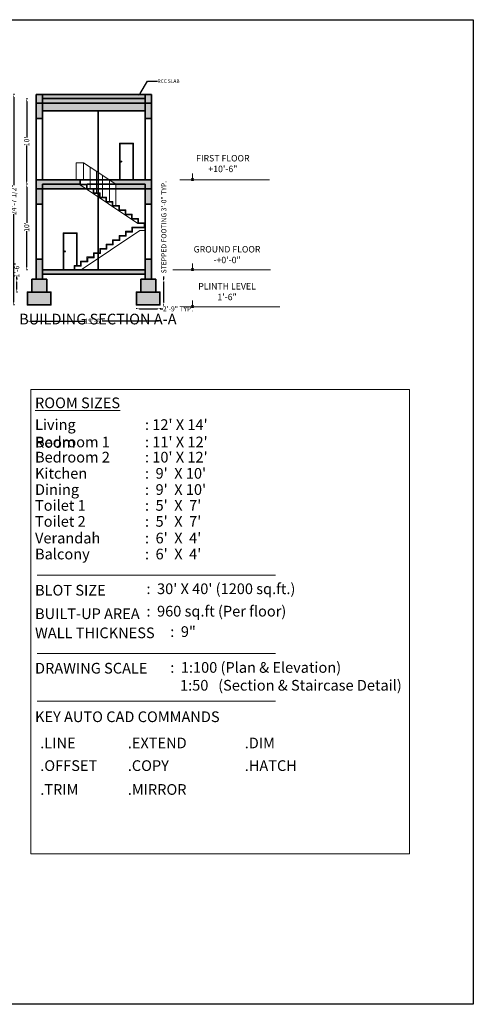
# Model space of a CAD drawing. Units: inches. Extents: x -80 to 1461, y -1239 to 153.
# Tile 6 of 6: x 824 to 1461, y -1239 to 141. Entities that reach past the tile are written whole.
import ezdxf
from ezdxf import colors
from ezdxf.entities.mleader import LeaderData, LeaderLine
from ezdxf.math import Vec2, Vec3

# ---------------------------------------------------------------- set-up
doc = ezdxf.new("R2010")
doc.units = ezdxf.units.IN
doc.header["$MEASUREMENT"] = 0
for name, color, linetype, lineweight in [('A-ANNO-DIMS', 2, 'Continuous', 18), ('A-ANNO-SYMB', 3, 'Continuous', 18), ('A-ANNO-TEXT', 7, 'Continuous', 18), ('A-ANNO-TTLB', 7, 'Continuous', 25), ('A-SECT', 7, 'Continuous', 35), ('A-SECT-PATT', 8, 'Continuous', 13), ('A-SECT-STRS', 7, 'Continuous', 20), ('DOOR', 32, 'Continuous', 18), ('S-FNDN', 7, 'Continuous', 35)]:
    doc.layers.add(name, color=color, linetype=linetype, lineweight=lineweight)
doc.styles.get("Standard").update_dxf_attribs({"font": 'arial.ttf'})
doc.dimstyles.get("Standard").update_dxf_attribs({"dimtxt": 7, "dimasz": 4, "dimexe": 0.18, "dimexo": 0.0625, "dimgap": 0.09, "dimtad": 0, "dimdec": 0, "dimzin": 0, "dimdsep": 46, "dimlunit": 3, "dimtxsty": 'Standard', "dimcen": 0.09, "dimadec": 0, "dimazin": 0, "dimtfac": 1, "dimtdec": 0, "dimtofl": 0, "dimtmove": 0, "dimatfit": 3, "dimfxl": 1, "dimfxlon": 1, "dimtolj": 1, "dimtzin": 0, "dimarcsym": 0})
pattern_1 = [(50, (-94.887, 315.974), (7.172602, -0.62752), [0.75, -8.25]), (355, (-94.887, 315.974), (-1.387513, 7.52192), [0.6, -6.6]), (100.45144, (-94.289, 315.9216), (5.78509, 6.8944), [0.6374, -7.01142]), (46.1842, (-94.887, 317.974), (10.672413, -1.65519), [1.125, -12.375]), (96.6356, (-93.998, 317.836), (9.34662, 9.74119), [0.9561, -10.51714]), (351.1842, (-94.887, 317.974), (9.34662, 9.74119), [0.9, -9.9]), (21, (-93.887, 317.474), (5.96907, -4.02619), [0.75, -8.25]), (326, (-93.887, 317.474), (2.433153, 7.2515), [0.6, -6.6]), (71.45144, (-93.3895, 317.1384), (8.402224, 3.22531), [0.6374, -7.01142]), (37.5, (-94.887, 315.974), (0.1215986, 3.3289385), [0, -6.52, 0, -6.7, 0, -6.625]), (7.5, (-94.887, 315.974), (2.630695, 3.944117), [0, -3.82, 0, -6.37, 0, -2.525]), (327.5, (-97.117, 315.974), (5.3382244, -0.225549), [0, -2.5, 0, -7.8, 0, -10.35]), (317.5, (-98.117, 315.974), (5.831862, 1.00105), [0, -3.25, 0, -5.18, 0, -7.35])]

# ---------------------------------------------------------------- blocks, each defined once
blk = doc.blocks.new('*D21')
at = {"layer": 'A-ANNO-DIMS', "color": 0, "lineweight": -2, "transparency": 16777216}
for p, q in [((820.2, -222.7), (820.2, -218.7)), ((821.2, -222.7), (820, -222.7)), ((820.2, -236.7), (820.2, -226.7)), ((821.2, -240.7), (820, -240.7))]:
    blk.add_line(p, q, dxfattribs=at)
at = {"layer": 'A-ANNO-DIMS', "color": 0, "transparency": 16777216}
for points in [[(819.5, -226.7), (820.9, -226.7), (820.2, -222.7)], [(819.5, -236.7), (820.9, -236.7), (820.2, -240.7)]]:
    blk.add_solid(points, dxfattribs=at)
at = {"layer": 'Defpoints', "color": 0, "transparency": 16777216}
for p in [(820.2, -222.7), (841.3, -222.7), (838.3, -240.7)]:
    blk.add_point(p, dxfattribs=at)
at = {"layer": 'A-ANNO-DIMS', "color": 0, "transparency": 16777216, "insert": (820.2, -209.6), "char_height": 7, "attachment_point": 5, "rotation": 90}
blk.add_mtext('\\A1;1\'-6"', dxfattribs=at)
blk = doc.blocks.new('*D22')
at = {"layer": 'A-ANNO-DIMS', "color": 0, "lineweight": -2, "transparency": 16777216}
for p, q in [((835.2, -89.4), (834, -89.4)), ((834.2, -93.4), (834.2, -143.7)), ((834.2, -205.4), (834.2, -155.1)), ((835.2, -209.4), (834, -209.4))]:
    blk.add_line(p, q, dxfattribs=at)
at = {"layer": 'A-ANNO-DIMS', "color": 0, "transparency": 16777216}
for points in [[(833.5, -93.4), (834.9, -93.4), (834.2, -89.4)], [(833.5, -205.4), (834.9, -205.4), (834.2, -209.4)]]:
    blk.add_solid(points, dxfattribs=at)
at = {"layer": 'Defpoints', "color": 0, "transparency": 16777216}
for p in [(834.2, -89.4), (856.3, -89.4), (856.3, -209.4)]:
    blk.add_point(p, dxfattribs=at)
at = {"layer": 'A-ANNO-DIMS', "color": 0, "transparency": 16777216, "insert": (834.2, -149.4), "char_height": 7, "attachment_point": 5, "rotation": 90}
blk.add_mtext("\\A1;10'", dxfattribs=at)
blk = doc.blocks.new('*D23')
at = {"layer": 'A-ANNO-DIMS', "color": 0, "lineweight": -2, "transparency": 16777216}
for p, q in [((835.2, 30.6), (834, 30.6)), ((834.2, 26.6), (834.2, -23.7)), ((834.2, -85.4), (834.2, -35.1)), ((835.2, -89.4), (834, -89.4))]:
    blk.add_line(p, q, dxfattribs=at)
at = {"layer": 'A-ANNO-DIMS', "color": 0, "transparency": 16777216}
for points in [[(833.5, 26.6), (834.9, 26.6), (834.2, 30.6)], [(833.5, -85.4), (834.9, -85.4), (834.2, -89.4)]]:
    blk.add_solid(points, dxfattribs=at)
at = {"layer": 'Defpoints', "color": 0, "transparency": 16777216}
for p in [(834.2, 30.6), (856.3, 30.6), (856.3, -89.4)]:
    blk.add_point(p, dxfattribs=at)
at = {"layer": 'A-ANNO-DIMS', "color": 0, "transparency": 16777216, "insert": (834.2, -29.4), "char_height": 7, "attachment_point": 5, "rotation": 90}
blk.add_mtext("\\A1;10'", dxfattribs=at)
blk = doc.blocks.new('FOOTING-STEPPED-SECTION')
blk.add_line((27, 36), (6, 36))
for points in [[(6, 36), (6, 18), (0, 18), (0, 0), (27, 0), (33, 0), (33, 18), (27, 18), (27, 36)], [(6, 18), (21, 18), (27, 18)]]:
    blk.add_lwpolyline(points)
blk = doc.blocks.new('LEVEL-DATUM')
h = blk.add_hatch(color=256)
h.dxf.hatch_style = 1
h.paths.add_polyline_path([(1.4, 2.8), (0, 2.8), (1.4, 1)])
h.paths.add_polyline_path([(2.8, 2.8), (1.4, 2.8), (1.4, 1)])
h = blk.add_hatch(color=256)
h.dxf.hatch_style = 1
h.paths.add_polyline_path([(2.8, 0), (2.8, 1), (0, 1), (0, 0)])
for p, q in [((1.4, 1), (0, 2.8)), ((0, 2.8), (1.4, 2.8)), ((0, 1), (2.8, 1)), ((0, 0), (0, 1)), ((2.8, 0), (0, 0)), ((1.4, 1), (1.4, 9.9)), ((1.4, 1), (2.8, 2.8)), ((2.8, 2.8), (1.4, 2.8)), ((2.8, 1), (2.8, 0))]:
    blk.add_line(p, q)
blk = doc.blocks.new('*D58')
at = {"layer": 'A-ANNO-DIMS', "color": 0, "lineweight": -2, "transparency": 16777216}
for p, q in [((1026.7, -222.7), (1026.7, -218.7)), ((1025.7, -222.7), (1026.8, -222.7)), ((1026.7, -254.7), (1026.7, -226.7)), ((1025.7, -258.7), (1026.8, -258.7))]:
    blk.add_line(p, q, dxfattribs=at)
at = {"layer": 'A-ANNO-DIMS', "color": 0, "transparency": 16777216}
for points in [[(1026, -226.7), (1027.3, -226.7), (1026.7, -222.7)], [(1026, -254.7), (1027.3, -254.7), (1026.7, -258.7)]]:
    blk.add_solid(points, dxfattribs=at)
at = {"layer": 'Defpoints', "color": 0, "transparency": 16777216}
for p in [(1021.3, -222.7), (1026.7, -222.7), (1021.3, -258.7)]:
    blk.add_point(p, dxfattribs=at)
at = {"layer": 'A-ANNO-DIMS', "color": 0, "transparency": 16777216, "insert": (1026.7, -149.5), "char_height": 7, "attachment_point": 5, "rotation": 90}
blk.add_mtext('\\A1;STEPPED FOOTING 3\'-0" TYP.', dxfattribs=at)
blk = doc.blocks.new('*D59')
at = {"layer": 'A-ANNO-DIMS', "color": 0, "lineweight": -2, "transparency": 16777216}
for p, q in [((988.3, -263.1), (988.3, -264.3)), ((992.3, -264.1), (1017.3, -264.1)), ((1021.3, -263.1), (1021.3, -264.3)), ((1021.3, -264.1), (1025.3, -264.1))]:
    blk.add_line(p, q, dxfattribs=at)
at = {"layer": 'A-ANNO-DIMS', "color": 0, "transparency": 16777216}
for points in [[(992.3, -263.4), (992.3, -264.7), (988.3, -264.1)], [(1017.3, -263.4), (1017.3, -264.7), (1021.3, -264.1)]]:
    blk.add_solid(points, dxfattribs=at)
at = {"layer": 'Defpoints', "color": 0, "transparency": 16777216}
for p in [(988.3, -258.7), (1021.3, -258.7), (1021.3, -264.1)]:
    blk.add_point(p, dxfattribs=at)
at = {"layer": 'A-ANNO-DIMS', "color": 0, "transparency": 16777216, "insert": (1046.7, -264.1), "char_height": 7, "attachment_point": 5}
blk.add_mtext('\\A1;2\'-9" TYP.', dxfattribs=at)
blk = doc.blocks.new('*D62')
at = {"layer": 'A-ANNO-DIMS', "color": 0, "lineweight": -2, "transparency": 16777216}
for p, q in [((835.3, -280.5), (835.3, -281.7)), ((839.3, -281.5), (916.5, -281.5)), ((1017.3, -281.5), (940, -281.5)), ((1021.3, -280.5), (1021.3, -281.7))]:
    blk.add_line(p, q, dxfattribs=at)
at = {"layer": 'A-ANNO-DIMS', "color": 0, "transparency": 16777216}
for points in [[(839.3, -280.8), (839.3, -282.2), (835.3, -281.5)], [(1017.3, -280.8), (1017.3, -282.2), (1021.3, -281.5)]]:
    blk.add_solid(points, dxfattribs=at)
at = {"layer": 'Defpoints', "color": 0, "transparency": 16777216}
for p in [(835.3, -258.7), (1021.3, -258.7), (1021.3, -281.5)]:
    blk.add_point(p, dxfattribs=at)
at = {"layer": 'A-ANNO-DIMS', "color": 0, "transparency": 16777216, "insert": (928.3, -281.5), "char_height": 7, "attachment_point": 5}
blk.add_mtext('\\A1;15\'-6"', dxfattribs=at)
blk = doc.blocks.new('*D63')
at = {"layer": 'A-ANNO-DIMS', "color": 0, "lineweight": -2, "transparency": 16777216}
for p, q in [((816.9, 36.6), (815.7, 36.6)), ((815.9, 32.6), (815.9, -90.7)), ((815.9, -254.7), (815.9, -131.3)), ((816.9, -258.7), (815.7, -258.7))]:
    blk.add_line(p, q, dxfattribs=at)
at = {"layer": 'A-ANNO-DIMS', "color": 0, "transparency": 16777216}
for points in [[(815.2, 32.6), (816.5, 32.6), (815.9, 36.6)], [(815.2, -254.7), (816.5, -254.7), (815.9, -258.7)]]:
    blk.add_solid(points, dxfattribs=at)
at = {"layer": 'Defpoints', "color": 0, "transparency": 16777216}
for p in [(815.9, 36.6), (847.3, 36.6), (835.3, -258.7)]:
    blk.add_point(p, dxfattribs=at)
at = {"layer": 'A-ANNO-DIMS', "color": 0, "transparency": 16777216, "insert": (815.9, -111), "char_height": 7, "attachment_point": 5, "rotation": 90}
blk.add_mtext('\\A1;24\'-7 1/2"', dxfattribs=at)
blk = doc.blocks.new('*D64')
at = {"layer": 'A-ANNO-DIMS', "color": 0, "lineweight": -2, "transparency": 16777216}
for p, q in [((847.3, -280.5), (847.3, -281.7)), ((851.3, -281.5), (916.5, -281.5)), ((1005.3, -281.5), (940, -281.5)), ((1009.3, -280.5), (1009.3, -281.7))]:
    blk.add_line(p, q, dxfattribs=at)
at = {"layer": 'A-ANNO-DIMS', "color": 0, "transparency": 16777216}
for points in [[(851.3, -280.8), (851.3, -282.2), (847.3, -281.5)], [(1005.3, -280.8), (1005.3, -282.2), (1009.3, -281.5)]]:
    blk.add_solid(points, dxfattribs=at)
at = {"layer": 'Defpoints', "color": 0, "transparency": 16777216}
for p in [(847.3, -222.7), (1009.3, -222.7), (1009.3, -281.5)]:
    blk.add_point(p, dxfattribs=at)
at = {"layer": 'A-ANNO-DIMS', "color": 0, "transparency": 16777216, "insert": (928.3, -281.5), "char_height": 7, "attachment_point": 5}
blk.add_mtext('\\A1;13\'-6"', dxfattribs=at)

msp = doc.modelspace()

# ---------------------------------------------------------------- hatches: boundary and pattern name
at = {"layer": 'A-SECT-PATT'}
h = msp.add_hatch(dxfattribs=at)
h.set_pattern_fill('AR-CONC', color=256)
h.set_pattern_definition(pattern_1)
h.paths.add_polyline_path([(856.26, 36.65), (847.26, 36.65), (847.26, 24.32), (856.26, 24.32)])
h.paths.add_polyline_path([(1000.26, 36.65), (957.78, 36.65), (909.26, 36.65), (856.26, 36.65), (856.26, 30.65), (909.26, 30.65), (919.26, 30.65), (961.99, 30.65), (1000.26, 30.65)])
h.paths.add_polyline_path([(1009.26, 36.65), (1000.26, 36.65), (1000.26, 30.65), (1000.26, 24.32), (1009.26, 24.32)])
h.paths.add_polyline_path([(1009.26, 24.32), (1000.26, 24.32), (1000.26, 2.65), (1009.26, 2.65)])
h.paths.add_polyline_path([(856.26, 24.32), (847.26, 24.32), (847.26, 2.65), (856.26, 2.65)])
h.paths.add_polyline_path([(909.26, -83.35), (847.26, -83.35), (847.26, -95.68), (856.26, -95.68), (856.26, -89.35), (909.26, -89.35)])
h.paths.add_polyline_path([(1009.26, -83.35), (957.78, -83.35), (950.26, -83.35), (959.26, -89.35), (961.99, -89.35), (1000.26, -89.35), (1000.26, -95.68), (1009.26, -95.68)])
h.paths.add_polyline_path([(1009.26, -95.68), (1000.26, -95.68), (1000.26, -117.35), (1009.26, -117.35)])
h.paths.add_polyline_path([(856.26, -95.68), (847.26, -95.68), (847.26, -117.35), (856.26, -117.35)])
h = msp.add_hatch(dxfattribs=at)
h.set_pattern_fill('AR-SAND', color=256)
h.set_pattern_definition([(37.5, (-94.8869, 315.974), (-0.0629934, 1.9268238), [0, -1.52, 0, -1.7, 0, -1.625]), (7.5, (-94.887, 315.974), (1.7697767, 2.822146), [0, -0.82, 0, -1.37, 0, -0.525]), (327.5, (-96.1169, 315.974), (3.1141419, 0.005659), [0, -0.5, 0, -1.8, 0, -2.35]), (317.5, (-96.117, 315.974), (3.0061266, 0.8776756), [0, -0.25, 0, -1.18, 0, -1.35])])
h.paths.add_polyline_path([(856.26, -89.35), (856.26, -95.68), (917.25, -95.68), (907.76, -89.35)])
h.paths.add_polyline_path([(959.26, -89.35), (959.26, -95.68), (1000.26, -95.68), (1000.26, -89.35)])
h.paths.add_polyline_path([(856.26, 30.65), (856.26, 24.32), (917.25, 24.32), (928.26, 24.32), (1000.26, 24.32), (1000.26, 30.65), (957.78, 30.65), (919.26, 30.65), (909.26, 30.65)])
h = msp.add_hatch(color=256, dxfattribs=at)
h.dxf.hatch_style = 1
h.set_gradient(color1=(199, 200, 202), name='CURVED')
h.paths.add_polyline_path([(917.25, 24.32), (856.26, 24.32), (856.26, 13.64), (1000.26, 13.64), (1000.26, 24.32), (928.26, 24.32)])
h = msp.add_hatch(dxfattribs=at)
h.set_pattern_fill('AR-CONC', color=256)
h.set_pattern_definition(pattern_1)
h.paths.add_polyline_path([(856.26, -194.45), (847.26, -194.45), (847.26, -222.68), (856.26, -222.68)])
h.paths.add_polyline_path([(1000.26, -209.35), (856.26, -209.35), (856.26, -215.35), (1000.26, -215.35)])
h.paths.add_polyline_path([(1009.26, -194.45), (1000.26, -194.45), (1000.26, -222.68), (1009.26, -222.68)])
h.paths.add_polyline_path([(1015.26, -222.68), (994.26, -222.68), (994.26, -240.68), (1009.26, -240.68), (1015.26, -240.68)])
h.paths.add_polyline_path([(1021.26, -240.68), (1015.26, -240.68), (1009.26, -240.68), (994.26, -240.68), (988.26, -240.68), (988.26, -258.68), (1015.26, -258.68), (1021.26, -258.68)])
h.paths.add_polyline_path([(868.26, -240.68), (862.26, -240.68), (856.26, -240.68), (841.26, -240.68), (835.26, -240.68), (835.26, -258.68), (862.26, -258.68), (868.26, -258.68)])
h.paths.add_polyline_path([(862.26, -222.68), (841.26, -222.68), (841.26, -240.68), (856.26, -240.68), (862.26, -240.68)])

# ---------------------------------------------------------------- linework, layer by layer
at = {"layer": 'A-ANNO-SYMB'}
for p, q in [((1048.99, -83.35), (1174.88, -83.35)), ((1039.22, -209.35), (1176.44, -209.35)), ((1053.18, -261.14), (1189.38, -261.14))]:
    msp.add_line(p, q, dxfattribs=at)
at = {"layer": 'A-ANNO-TEXT'}
for p, q in [((848.85, -637.34), (1183.38, -637.34)), ((848.85, -747.4), (1183.38, -747.4)), ((848.85, -814.34), (1183.38, -814.34))]:
    msp.add_line(p, q, dxfattribs=at)
msp.add_lwpolyline([(840.02, -377.35), (1371.71, -377.35), (1371.71, -1028.24), (840.02, -1028.24)], close=True, dxfattribs=at)
at = {"layer": 'A-ANNO-TTLB'}
msp.add_lwpolyline([(-79.81, 141.36), (1461.09, 141.36), (1461.09, -1239.28), (-79.81, -1239.28)], close=True, dxfattribs=at)
at = {"layer": 'A-SECT'}
for p, q in [((847.26, -222.68), (847.26, 36.65)), ((909.26, 36.65), (847.26, 36.65)), ((856.26, -83.35), (856.26, 36.65)), ((909.26, 30.65), (856.26, 30.65)), ((957.78, 36.65), (909.26, 36.65)), ((919.26, 30.65), (909.26, 30.65)), ((919.26, 30.65), (961.99, 30.65)), ((1009.26, 36.65), (957.78, 36.65)), ((1000.26, 30.65), (957.78, 30.65)), ((1000.26, -83.35), (1000.26, 36.65)), ((1009.26, -222.68), (1009.26, 36.65)), ((847.26, 24.32), (917.25, 24.32)), ((928.26, 24.32), (917.25, 24.32)), ((928.26, 24.32), (1009.26, 24.32)), ((856.26, 2.65), (847.26, 2.65)), ((856.26, 13.64), (1000.26, 13.64)), ((934.32, -209.35), (934.32, 13.64)), ((1009.26, 2.65), (1000.26, 2.65)), ((909.26, -83.35), (847.26, -83.35)), ((847.26, -95.68), (917.25, -95.68)), ((856.26, -222.68), (856.26, -89.35)), ((909.26, -89.35), (856.26, -89.35)), ((957.78, -83.35), (909.26, -83.35)), ((909.26, -89.35), (909.26, -83.35)), ((919.26, -89.35), (961.99, -89.35)), ((928.26, -95.68), (1009.26, -95.68)), ((1009.26, -83.35), (957.78, -83.35)), ((1000.26, -89.35), (957.78, -89.35)), ((1000.26, -222.68), (1000.26, -89.35)), ((856.26, -117.35), (847.26, -117.35)), ((1009.26, -117.35), (1000.26, -117.35)), ((856.26, -209.35), (1000.26, -209.35)), ((856.26, -215.35), (1000.26, -215.35))]:
    msp.add_line(p, q, dxfattribs=at)
at = {"layer": 'A-SECT-STRS'}
for p, q in [((903.7, -83.35), (903.7, -59.14)), ((913.94, -59.14), (903.7, -59.14)), ((923.26, -65.35), (913.94, -59.14)), ((913.94, -59.14), (913.94, -83.35)), ((923.26, -95.35), (923.26, -65.35)), ((959.26, -89.35), (923.26, -65.35)), ((932.26, -101.35), (932.26, -71.35)), ((940.76, -107.35), (940.76, -77.35)), ((907.76, -89.35), (990.26, -144.35)), ((919.26, -89.35), (909.26, -89.35)), ((909.26, -89.35), (909.26, -90.35)), ((909.26, -90.35), (918.26, -90.35)), ((918.26, -90.35), (918.26, -95.35)), ((918.26, -95.35), (918.26, -96.35)), ((918.26, -96.35), (927.26, -96.35)), ((919.26, -95.35), (919.26, -89.35)), ((928.26, -95.35), (919.26, -95.35)), ((927.26, -96.35), (927.26, -101.35)), ((928.26, -101.35), (928.26, -95.35)), ((950.26, -113.35), (950.26, -83.35)), ((959.26, -119.35), (959.26, -89.35)), ((927.26, -101.35), (927.26, -102.35)), ((927.26, -102.35), (936.26, -102.35)), ((937.26, -101.35), (928.26, -101.35)), ((936.26, -102.35), (936.26, -107.35)), ((946.26, -107.35), (936.26, -107.35)), ((936.26, -107.35), (936.26, -108.35)), ((936.26, -108.35), (945.26, -108.35)), ((937.26, -107.35), (937.26, -101.35)), ((945.26, -108.35), (945.26, -113.35)), ((946.26, -113.35), (946.26, -107.35)), ((955.26, -113.35), (945.26, -113.35)), ((945.26, -113.35), (945.26, -114.35)), ((945.26, -114.35), (954.26, -114.35)), ((954.26, -114.35), (954.26, -119.35)), ((964.26, -119.35), (954.26, -119.35)), ((954.26, -119.35), (954.26, -120.35)), ((954.26, -120.35), (963.26, -120.35)), ((955.26, -119.35), (955.26, -113.35)), ((963.26, -120.35), (963.26, -125.35)), ((964.26, -125.35), (964.26, -119.35)), ((973.26, -125.35), (963.26, -125.35)), ((963.26, -125.35), (963.26, -126.35)), ((963.26, -126.35), (972.26, -126.35)), ((972.26, -126.35), (972.26, -131.35)), ((982.26, -131.35), (972.26, -131.35)), ((972.26, -131.35), (972.26, -132.35)), ((972.26, -132.35), (981.26, -132.35)), ((973.26, -131.35), (973.26, -125.35)), ((981.26, -132.35), (981.26, -137.35)), ((991.26, -137.35), (981.26, -137.35)), ((981.26, -137.35), (981.26, -138.35)), ((982.26, -137.35), (982.26, -131.35)), ((991.26, -143.35), (991.26, -137.35)), ((981.26, -138.35), (990.26, -138.35)), ((981.74, -155.35), (981.74, -149.35)), ((981.74, -149.35), (999.26, -149.35)), ((1000.26, -150.35), (982.74, -150.35)), ((982.74, -150.35), (982.74, -155.35)), ((990.26, -138.35), (990.26, -143.35)), ((1000.26, -143.35), (990.26, -143.35)), ((990.26, -143.35), (990.26, -144.35)), ((990.26, -144.35), (999.26, -144.35)), ((999.26, -144.35), (999.26, -149.35)), ((999.26, -149.35), (1000.26, -149.35)), ((1000.26, -149.35), (1000.26, -143.35)), ((1000.26, -150.35), (1000.26, -154.35)), ((963.74, -167.35), (963.74, -161.35)), ((963.74, -161.35), (973.74, -161.35)), ((973.74, -162.35), (964.74, -162.35)), ((964.74, -162.35), (964.74, -167.35)), ((972.74, -161.35), (972.74, -155.35)), ((972.74, -155.35), (982.74, -155.35)), ((982.74, -156.35), (973.74, -156.35)), ((973.74, -156.35), (973.74, -161.35)), ((973.74, -161.35), (973.74, -162.35)), ((982.74, -155.35), (982.74, -156.35)), ((1000.26, -154.35), (992.95, -154.35)), ((936.74, -185.35), (936.74, -179.35)), ((936.74, -179.35), (946.74, -179.35)), ((945.74, -179.35), (945.74, -173.35)), ((945.74, -173.35), (955.74, -173.35)), ((955.74, -174.35), (946.74, -174.35)), ((946.74, -174.35), (946.74, -179.35)), ((946.74, -179.35), (946.74, -180.35)), ((954.74, -173.35), (954.74, -167.35)), ((954.74, -167.35), (964.74, -167.35)), ((964.74, -168.35), (955.74, -168.35)), ((955.74, -168.35), (955.74, -173.35)), ((955.74, -173.35), (955.74, -174.35)), ((964.74, -167.35), (964.74, -168.35)), ((918.74, -197.35), (918.74, -191.35)), ((918.74, -191.35), (928.74, -191.35)), ((928.74, -192.35), (919.74, -192.35)), ((919.74, -192.35), (919.74, -197.35)), ((927.74, -191.35), (927.74, -185.35)), ((927.74, -185.35), (937.74, -185.35)), ((937.74, -186.35), (928.74, -186.35)), ((928.74, -186.35), (928.74, -191.35)), ((928.74, -191.35), (928.74, -192.35)), ((946.74, -180.35), (937.74, -180.35)), ((937.74, -180.35), (937.74, -185.35)), ((937.74, -185.35), (937.74, -186.35)), ((900.74, -209.35), (900.74, -203.35)), ((900.74, -203.35), (910.74, -203.35)), ((910.74, -204.35), (901.74, -204.35)), ((901.74, -204.35), (901.74, -209.35)), ((909.74, -203.35), (909.74, -197.35)), ((909.74, -197.35), (919.74, -197.35)), ((919.74, -198.35), (910.74, -198.35)), ((910.74, -198.35), (910.74, -203.35)), ((910.74, -203.35), (910.74, -204.35)), ((919.74, -197.35), (919.74, -198.35)), ((901.74, -209.35), (900.74, -209.35))]:
    msp.add_line(p, q, dxfattribs=at)
msp.add_lwpolyline([(992.95, -154.35), (910.45, -209.35)], dxfattribs=at)
at = {"layer": 'DOOR'}
for points in [[(983.96, -83.35), (964.39, -83.35), (964.39, -31.61), (983.96, -31.61), (983.96, -83.35)], [(965.39, -83.35), (965.39, -32.61), (982.96, -32.61), (982.96, -83.35)], [(904.85, -209.35), (885.28, -209.35), (885.28, -157.61), (904.85, -157.61), (904.85, -203.35)], [(886.28, -209.35), (886.28, -158.61), (903.85, -158.61), (903.85, -203.35)]]:
    msp.add_lwpolyline(points, dxfattribs=at)
for centre in [(966.97, -57.53), (887.86, -183.53)]:
    msp.add_circle(centre, 0.724, dxfattribs=at)
at = {"layer": 'S-FNDN'}
for p, q in [((847.26, -194.45), (856.26, -194.45)), ((1000.26, -194.45), (1009.26, -194.45))]:
    msp.add_line(p, q, dxfattribs=at)

# ---------------------------------------------------------------- block references
at = {"layer": 'A-ANNO-SYMB'}
for p in [(1065.31, -84.31), (1065.7, -210.31), (1065.7, -262.1)]:
    msp.add_blockref('LEVEL-DATUM', p, dxfattribs=at)
at = {"layer": 'S-FNDN'}
for p in [(835.26, -258.68), (988.26, -258.68)]:
    msp.add_blockref('FOOTING-STEPPED-SECTION', p, dxfattribs=at)

# ---------------------------------------------------------------- texts
at = {"layer": 'A-ANNO-SYMB', "char_height": 9, "attachment_point": 1}
for s, width, insert in [('\\pxqc;FIRST FLOOR\\P+10\'-6"', 96.7224, (1061.15, -48.41)), ('\\pxqc;GROUND FLOOR\\P-+0\'-0"', 108.4526, (1061.15, -176.07)), ('\\pxqc;PLINTH LEVEL\\P1\'-6"', 108.4526, (1061.15, -227.99))]:
    msp.add_mtext_dynamic_manual_height_columns(s, width=width, gutter_width=1, heights=[0], dxfattribs=dict(at, insert=insert))
at = {"layer": 'A-ANNO-TEXT', "char_height": 15, "attachment_point": 1}
for s, width, insert in [('\\pxqc;BUILDING SECTION A-A', 245.0183, (811.56, -270.94)), ('{\\fArial|b1|i0|c0|p34;\\LROOM SIZES}', 245.0183, (845.84, -388.43)), ('Living Room', 116.7938, (845.84, -418.91)), (": 12' X 14'", 116.7938, (1000.18, -418.91)), ('Bedroom 1', 116.7938, (845.84, -443.25)), (": 11' X 12'", 116.7938, (1000.18, -443.25)), ('Bedroom 2', 116.7938, (845.84, -464.56)), (": 10' X 12'", 116.7938, (1000.18, -464.56)), ('Kitchen', 116.7938, (845.84, -487.27)), (":  9'  X 10'", 116.7938, (1000.18, -487.27)), ('Dining', 116.7938, (845.84, -509.99)), (":  9'  X 10'", 116.7938, (1000.18, -509.99)), ('Toilet 1', 116.7938, (845.84, -532.2)), (":  5'  X  7'", 116.7938, (1000.18, -532.2)), ('Toilet 2', 116.7938, (845.84, -554.62)), (":  5'  X  7'", 116.7938, (1000.18, -554.62)), ('Verandah', 116.7938, (845.84, -578.01)), (":  6'  X  4'", 116.7938, (1000.18, -578.01)), ('Balcony', 116.7938, (845.84, -600.42)), (":  6'  X  4'", 116.7938, (1000.18, -600.42)), (":  30' X 40' (1200 sq.ft.)", 240.1081, (1002.27, -649.09)), ('BLOT SIZE', 110.3298, (845.84, -651.14)), ('BUILT-UP AREA', 159.7477, (845.84, -684.1)), (':  960 sq.ft (Per floor)', 240.1081, (1002.27, -680.51)), ('WALL THICKNESS', 183.3709, (845.84, -710.92)), (':  9"', 45.3861, (1035.68, -709.16)), (':  1:100 (Plan & Elevation)\\P   1:50   (Section & Staircase Detail)', 341.2875, (1035.68, -759.42)), ('DRAWING SCALE', 180.1783, (845.84, -760.52)), ('KEY AUTO CAD COMMANDS', 306.8439, (845.84, -828.57)), ('.LINE', 45.3861, (853.19, -865.34)), ('.EXTEND', 45.3861, (976.04, -865.34)), ('.DIM', 45.3861, (1140.2, -865.34)), ('.OFFSET', 45.3861, (853.19, -897.1)), ('.COPY', 45.3861, (976.04, -897.1)), ('.HATCH', 45.3861, (1140.2, -897.1)), ('.TRIM', 45.3861, (853.19, -930.55)), ('.MIRROR', 45.3861, (976.04, -930.55))]:
    msp.add_mtext_dynamic_manual_height_columns(s, width=width, gutter_width=1, heights=[0], dxfattribs=dict(at, insert=insert))

# ---------------------------------------------------------------- dimensions: what is measured, and where the dimension line sits
at = {"layer": 'A-ANNO-DIMS'}
for base, p1, p2, override, picture, middle in [((815.86, 36.65), (835.26, -258.68), (847.26, 36.65), {"dimdec": 1, "dimlfac": 1, "dimrnd": 0, "dimzin": 1, "dimdsep": 46, "dimlunit": 4, "dimfrac": 2}, '*D63', (815.86, -111.02)), ((834.21, 30.65), (856.26, -89.35), (856.26, 30.65), {"dimclrd": 0, "dimclre": 0, "dimclrt": 0}, '*D23', (834.21, -29.35)), ((834.21, -89.35), (856.26, -209.35), (856.26, -89.35), {"dimclrd": 0, "dimclre": 0, "dimclrt": 0}, '*D22', (834.21, -149.35)), ((820.21, -222.68), (838.26, -240.68), (841.26, -222.68), {"dimclrd": 0, "dimclre": 0, "dimclrt": 0}, '*D21', (820.21, -209.62))]:
    dim = msp.add_linear_dim(base=base, p1=p1, p2=p2, angle=90, dimstyle='Standard', override=override, dxfattribs=at)
    dim.commit()
    dim.dimension.update_dxf_attribs({"geometry": picture, "text_midpoint": middle})
dim = msp.add_linear_dim(base=(1026.66, -222.68), p1=(1021.26, -258.68), p2=(1021.26, -222.68), angle=90, text='STEPPED FOOTING <> TYP.', dimstyle='Standard', override={"dimdec": 1, "dimlfac": 1, "dimrnd": 0, "dimzin": 1, "dimdsep": 46, "dimlunit": 4, "dimfrac": 2}, dxfattribs=at)
dim.commit()
dim.dimension.update_dxf_attribs({"geometry": '*D58', "text_midpoint": (1026.66, -149.46)})
for base, p1, p2, picture in [((1009.26, -281.5), (847.26, -222.68), (1009.26, -222.68), '*D64'), ((1021.26, -281.5), (835.26, -258.68), (1021.26, -258.68), '*D62')]:
    dim = msp.add_linear_dim(base=base, p1=p1, p2=p2, dimstyle='Standard', override={"dimdec": 1, "dimlfac": 1, "dimrnd": 0, "dimzin": 1, "dimdsep": 46, "dimlunit": 4, "dimfrac": 2}, dxfattribs=at)
    dim.commit()
    dim.dimension.update_dxf_attribs({"geometry": picture, "text_midpoint": (928.26, -281.5)})
dim = msp.add_linear_dim(base=(1021.26, -264.08), p1=(988.26, -258.68), p2=(1021.26, -258.68), text='<> TYP.', dimstyle='Standard', override={"dimdec": 1, "dimlfac": 1, "dimrnd": 0, "dimzin": 1, "dimdsep": 46, "dimlunit": 4, "dimfrac": 2}, dxfattribs=at)
dim.commit()
dim.dimension.update_dxf_attribs({"geometry": '*D59', "text_midpoint": (1046.75, -264.08)})

# ---------------------------------------------------------------- leaders
at = {"layer": 'A-ANNO-TEXT'}
ml = msp.add_multileader_mtext('Standard', dxfattribs=at)
ml.set_content('RCC SLAB', color=256)
ml.set_leader_properties()
ml.build(insert=Vec2(0, 0))
ml.multileader.update_dxf_attribs({"dogleg_length": 0.36})
ctx = ml.context
ctx.base_point, ctx.char_height, ctx.landing_gap_size, ctx.plane_origin = Vec3(1017.66, 55.13), 5, 0.09, Vec3(991.41, 34.35)
notes = []
notes.append((ctx, [(0, (1, 1, 0), (1017.3, 55.13), (1, 0), 0.36, [(0, [(991.41, 34.35), (1003.89, 55.13)], 0, [])])]))
ctx.mtext.insert, ctx.mtext.flow_direction = Vec3(1017.75, 57.67), 5
for ctx, leaders in notes:
    for number, flags, end, landing, length, lines in leaders:
        leader = LeaderData()
        leader.index, (leader.has_last_leader_line, leader.has_dogleg_vector, leader.attachment_direction) = number, flags
        leader.last_leader_point, leader.dogleg_vector, leader.dogleg_length = Vec3(end), Vec3(landing), length
        for number, points, colour, breaks in lines:
            line = LeaderLine()
            line.index, line.vertices, line.color, line.breaks = number, Vec3.list(points), colors.encode_raw_color(colour), breaks
            leader.lines.append(line)
        ctx.leaders.append(leader)

doc.saveas('drawing.dxf')
